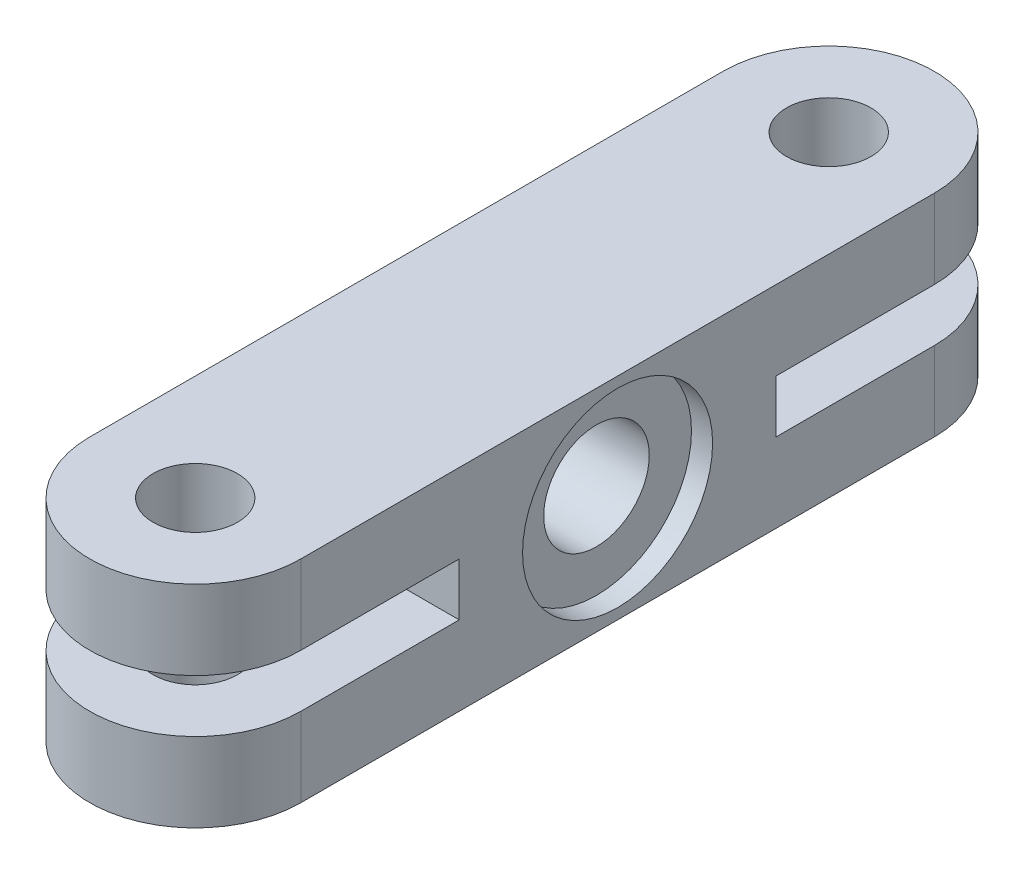
from build123d import *

# Parameters (mm, degrees)
LINK_BODY_DEPTH        = 10
PIN_HOLES_SKETCH_R     = 4
PIN_HOLES_2X_8_DEPTH   = 10
SIDE_SLOTS_SKETCH_R    = 5
SIDE_SLOTS_SKETCH_W    = 30.75281097
SIDE_SLOTS_SKETCH_H    = 5
SIDE_SLOTS_SKETCH_W_2  = 29.537366276
SIDE_SLOTS_CUT_DEPTH   = 10
COUNTERBORE_SKETCH_R   = 9
COUNTERBORE_18X2_DEPTH = 2


with BuildPart() as part:
    # Link Body Sketch → Link Body (new, symmetric)
    with BuildSketch(Plane(origin=(0, 0, 0), x_dir=(1, 0, 0), z_dir=(0, 1, 0))):
        with BuildLine():
            Line((10, 30), (10, -30))
            ThreePointArc((10, -30), (0, -40), (-10, -30))
            Line((-10, -30), (-10, 30))
            ThreePointArc((-10, 30), (0, 40), (10, 30))
        make_face()
    extrude(amount=LINK_BODY_DEPTH, both=True)

    # Pin Holes Sketch → Pin Holes 2xØ8 (cut, symmetric)
    with BuildSketch(Plane(origin=(0, 0, 0), x_dir=(1, 0, 0), z_dir=(0, 1, 0))):
        with Locations(Location((0, 30, 0), (0, 0, 270))):
            Circle(PIN_HOLES_SKETCH_R)
        with Locations(Location((0, -30, 0), (0, 0, 270))):
            Circle(PIN_HOLES_SKETCH_R)
    extrude(amount=PIN_HOLES_2X_8_DEPTH, both=True, mode=Mode.SUBTRACT)

    # Side Slots Sketch → Side Slots Cut (cut, symmetric)
    with BuildSketch(Plane(origin=(0, 0, 0), x_dir=(0, 0, -1), z_dir=(1, 0, 0))):
        Circle(SIDE_SLOTS_SKETCH_R)
        with Locations((-30.376405485, 0)):
            Rectangle(SIDE_SLOTS_SKETCH_W, SIDE_SLOTS_SKETCH_H)
        with Locations((29.768683138, 0)):
            Rectangle(SIDE_SLOTS_SKETCH_W_2, SIDE_SLOTS_SKETCH_H)
    extrude(amount=SIDE_SLOTS_CUT_DEPTH, both=True, mode=Mode.SUBTRACT)

    # Counterbore Sketch → Counterbore Ø18x2 (cut)
    with BuildSketch(Plane(origin=(10, 0, 0), x_dir=(0, 0, -1), z_dir=(1, 0, 0))):
        Circle(COUNTERBORE_SKETCH_R)
    extrude(amount=-COUNTERBORE_18X2_DEPTH, mode=Mode.SUBTRACT)


solid = part.part
